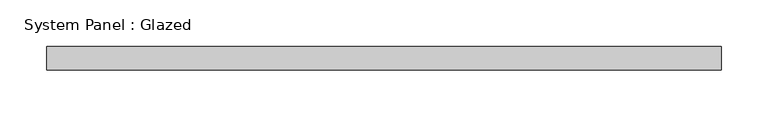
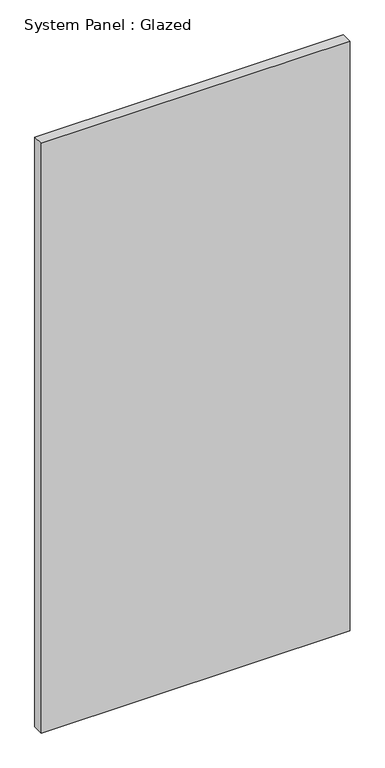
"""IFC4 building model written with IfcOpenShell, lengths in millimetres: plate geometry, System Panel : Glazed."""

from ifc_helpers import new_model, si_unit, origin, origin_with_axes, place, context, project, spatial, polyline, outline, extrude, source, transform, mapped, element, save


def system_panel_glazed_9d0e0944(model_context):
    return source(origin(), model_context, "Body", "SweptSolid", [
        extrude(outline(polyline([(362.0017238, 19.05), (-362.0017238, 19.05), (-362.0017238, 44.45), (362.0017238, 44.45), (362.0017238, 19.05)])), origin_with_axes(), (0.0, 0.0, 1.0), 1460.5),
    ])


if __name__ == "__main__":
    model = new_model("IFC4")
    model_context = context("Model", 3, world=origin())
    ifc_project = project(units=[si_unit("LENGTHUNIT", "METRE", prefix="MILLI")], contexts=[model_context])
    site = spatial("IfcSite", under=ifc_project)
    building = spatial("IfcBuilding", under=site)
    placement = place(None, origin())
    system_panel_glazed_shape = system_panel_glazed_9d0e0944(model_context)
    element("IfcPlate", 1, ObjectType="System Panel : Glazed", at=placement, inside=building, context=model_context, shape_type="MappedRepresentation", body=[
        mapped(system_panel_glazed_shape, transform((0.0, 0.0, 0.0), x_axis=(1.0, 0.0, 0.0), y_axis=(0.0, 1.0, 0.0), z_axis=(0.0, 0.0, 1.0))),
    ])
    save(model, "model.ifc")

# Revit data of these elements
# Type "System Panel : Glazed"
#   Construction Type Id = "GSP4R"
#   Analytic Construction = "1/8 in Pilkington single glazing"
#   Visual Light Transmittance = 0.9
#   Solar Heat Gain Coefficient = 0.86
#   Heat Transfer Coefficient (U) = 1.18115 BTU/(h·ft²·°F)
#   Define Thermal Properties by = 1
# Element 1 (IfcPlate, "System Panel : Glazed")
#   Materials on its faces: "Glass"
# Materials
#   "Glass": class "Glass", colour RGB 0 128 192, transparency 0.75, Description = "Soda Lime Glass", Cost = 0
